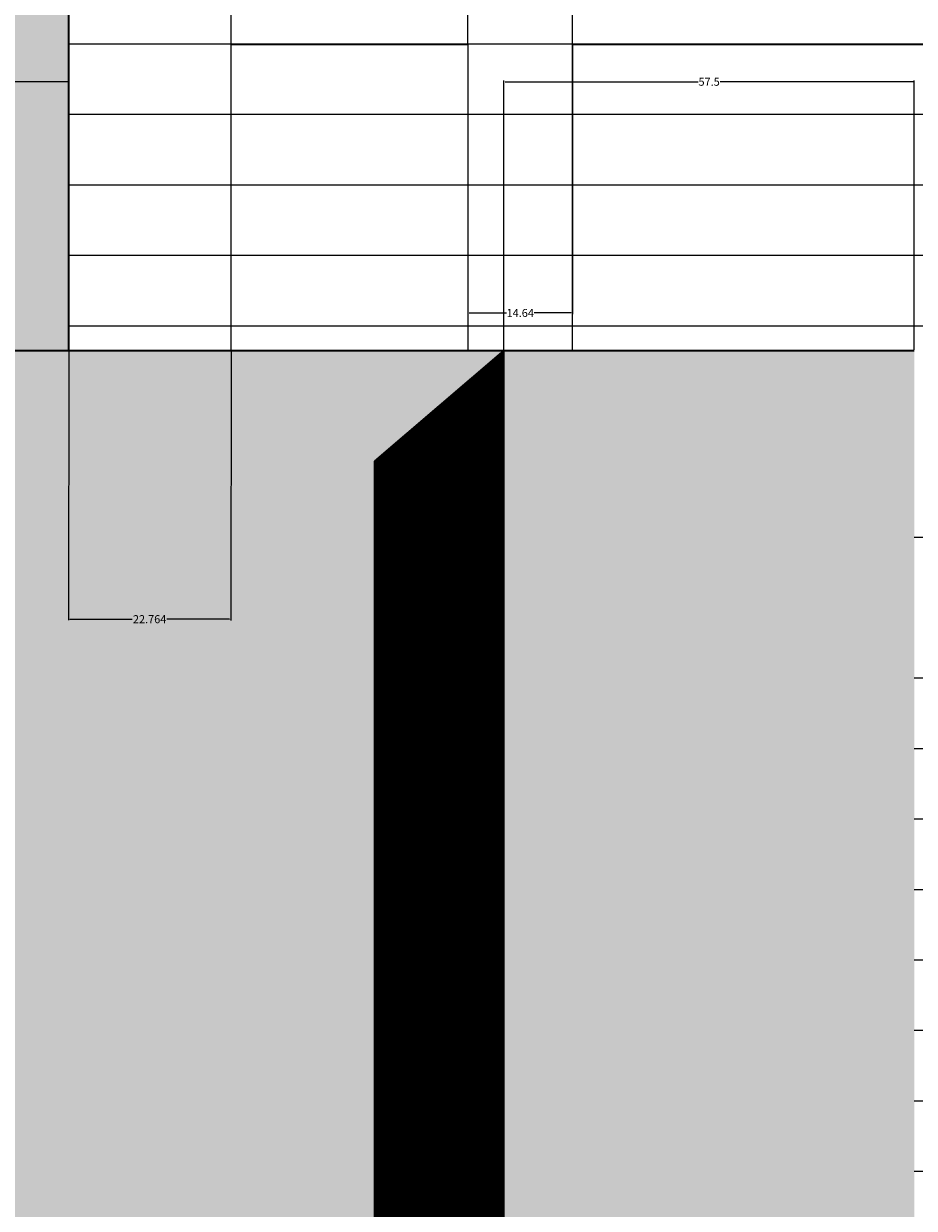
# Model space of a CAD drawing. Units: inches. Extents: x 8 to 634, y 41 to 867.
# Tile 18 of 21: x 293 to 418, y 577 to 743. Entities that reach past the tile are written whole.
import ezdxf

# ---------------------------------------------------------------- set-up
doc = ezdxf.new("R2010")
doc.units = ezdxf.units.IN
doc.header["$MEASUREMENT"] = 0
for name, color, linetype, lineweight in [('A-ANNO-DIMS', 2, 'Continuous', 18), ('A-ELEV-PATT', 252, 'Continuous', 9), ('A-GLAZ', 4, 'Continuous', 25), ('A-ROOF', 7, 'Continuous', 35), ('A-ROOF-PATT', 8, 'Continuous', 9), ('A-WALL', 7, 'Continuous', 35), ('A-WALL-PATT', 8, 'Continuous', 9)]:
    doc.layers.add(name, color=color, linetype=linetype, lineweight=lineweight)
doc.layers.add('A-GLAZ-PATT', color=251, linetype='Continuous', lineweight=9, true_color=0x636466)
doc.styles.get("Standard").update_dxf_attribs({"font": 'arial.ttf'})
doc.dimstyles.get("Standard").update_dxf_attribs({"dimtxt": 1.125, "dimasz": 0.18, "dimexe": 0.18, "dimexo": 0.0625, "dimgap": 0.09, "dimtad": 0, "dimtih": 1, "dimtoh": 1, "dimdec": 4, "dimzin": 0, "dimdsep": 46, "dimlunit": 4, "dimtxsty": 'Standard', "dimcen": 0.09, "dimadec": 0, "dimazin": 0, "dimtfac": 1, "dimtdec": 4, "dimtofl": 0, "dimtmove": 0, "dimatfit": 3, "dimfxl": 1, "dimtolj": 1, "dimtzin": 0, "dimarcsym": 0})

# ---------------------------------------------------------------- blocks, each defined once
blk = doc.blocks.new('*D19')
at = {"layer": 'A-ANNO-DIMS', "color": 0, "lineweight": -2, "transparency": 16777216}
for p, q in [((47.34, 697.73), (47.34, 866.81)), ((594.35, 827.83), (594.35, 866.81)), ((47.52, 866.63), (319.51, 866.63)), ((594.17, 866.63), (322.18, 866.63))]:
    blk.add_line(p, q, dxfattribs=at)
at = {"layer": 'A-ANNO-DIMS', "color": 0, "transparency": 16777216}
for points in [[(47.52, 866.66), (47.52, 866.6), (47.34, 866.63)], [(594.17, 866.66), (594.17, 866.6), (594.35, 866.63)]]:
    blk.add_solid(points, dxfattribs=at)
at = {"layer": 'Defpoints', "color": 0, "transparency": 16777216}
for p in [(594.35, 866.63), (594.35, 827.77), (47.34, 697.67)]:
    blk.add_point(p, dxfattribs=at)
at = {"layer": 'A-ANNO-DIMS', "color": 0, "transparency": 16777216, "insert": (320.85, 866.63), "char_height": 1.125, "attachment_point": 5}
blk.add_mtext('\\A1;547', dxfattribs=at)
blk = doc.blocks.new('*D24')
at = {"layer": 'A-ANNO-DIMS', "color": 0, "lineweight": -2, "transparency": 16777216}
for p, q in [((262.23, 697.73), (262.23, 735.5)), ((299.8, 697.73), (299.8, 735.5)), ((262.41, 735.32), (279.02, 735.32)), ((299.62, 735.32), (283, 735.32))]:
    blk.add_line(p, q, dxfattribs=at)
at = {"layer": 'A-ANNO-DIMS', "color": 0, "transparency": 16777216}
for points in [[(262.41, 735.35), (262.41, 735.29), (262.23, 735.32)], [(299.62, 735.35), (299.62, 735.29), (299.8, 735.32)]]:
    blk.add_solid(points, dxfattribs=at)
at = {"layer": 'Defpoints', "color": 0, "transparency": 16777216}
for p in [(299.8, 735.32), (262.23, 697.67), (299.8, 697.67)]:
    blk.add_point(p, dxfattribs=at)
at = {"layer": 'A-ANNO-DIMS', "color": 0, "transparency": 16777216, "insert": (281.01, 735.32), "char_height": 1.125, "attachment_point": 5}
blk.add_mtext('\\A1;37.57', dxfattribs=at)
blk = doc.blocks.new('*D25')
at = {"layer": 'A-ANNO-DIMS', "color": 0, "lineweight": -2, "transparency": 16777216}
for p, q in [((299.8, 697.6), (299.76, 659.84)), ((322.56, 697.58), (322.52, 659.81)), ((299.94, 660.02), (308.71, 660.01)), ((322.34, 659.99), (313.57, 660))]:
    blk.add_line(p, q, dxfattribs=at)
at = {"layer": 'A-ANNO-DIMS', "color": 0, "transparency": 16777216}
for points in [[(299.94, 660.05), (299.94, 659.99), (299.76, 660.02)], [(322.34, 660.02), (322.34, 659.96), (322.52, 659.99)]]:
    blk.add_solid(points, dxfattribs=at)
at = {"layer": 'Defpoints', "color": 0, "transparency": 16777216}
for p in [(299.8, 697.67), (322.56, 697.64), (299.76, 660.02)]:
    blk.add_point(p, dxfattribs=at)
at = {"layer": 'A-ANNO-DIMS', "color": 0, "transparency": 16777216, "insert": (311.14, 660), "char_height": 1.125, "attachment_point": 5}
blk.add_mtext('\\A1;22.764', dxfattribs=at)
blk = doc.blocks.new('*D48')
at = {"layer": 'A-ANNO-DIMS', "color": 0, "lineweight": -2, "transparency": 16777216}
for p, q in [((322.56, 740.62), (322.56, 778.39)), ((322.74, 778.21), (336.73, 778.21)), ((355.57, 778.21), (341.58, 778.21)), ((355.75, 740.62), (355.75, 778.39))]:
    blk.add_line(p, q, dxfattribs=at)
at = {"layer": 'A-ANNO-DIMS', "color": 0, "transparency": 16777216}
for points in [[(322.74, 778.24), (322.74, 778.18), (322.56, 778.21)], [(355.57, 778.24), (355.57, 778.18), (355.75, 778.21)]]:
    blk.add_solid(points, dxfattribs=at)
at = {"layer": 'Defpoints', "color": 0, "transparency": 16777216}
for p in [(355.75, 778.21), (322.56, 740.56), (355.75, 740.56)]:
    blk.add_point(p, dxfattribs=at)
at = {"layer": 'A-ANNO-DIMS', "color": 0, "transparency": 16777216, "insert": (339.15, 778.21), "char_height": 1.125, "attachment_point": 5}
blk.add_mtext('\\A1;33.187', dxfattribs=at)
blk = doc.blocks.new('*D49')
at = {"layer": 'A-ANNO-DIMS', "color": 0, "lineweight": -2, "transparency": 16777216}
for p, q in [((355.75, 740.49), (355.75, 702.73)), ((370.39, 740.49), (370.39, 702.73)), ((355.93, 702.91), (361.13, 702.91)), ((370.21, 702.91), (365, 702.91))]:
    blk.add_line(p, q, dxfattribs=at)
at = {"layer": 'A-ANNO-DIMS', "color": 0, "transparency": 16777216}
for points in [[(355.93, 702.94), (355.93, 702.88), (355.75, 702.91)], [(370.21, 702.94), (370.21, 702.88), (370.39, 702.91)]]:
    blk.add_solid(points, dxfattribs=at)
at = {"layer": 'Defpoints', "color": 0, "transparency": 16777216}
for p in [(355.75, 740.56), (370.39, 740.56), (355.75, 702.91)]:
    blk.add_point(p, dxfattribs=at)
at = {"layer": 'A-ANNO-DIMS', "color": 0, "transparency": 16777216, "insert": (363.07, 702.91), "char_height": 1.125, "attachment_point": 5}
blk.add_mtext('\\A1;14.64', dxfattribs=at)
blk = doc.blocks.new('*D50')
at = {"layer": 'A-ANNO-DIMS', "color": 0, "lineweight": -2, "transparency": 16777216}
for p, q in [((370.39, 740.62), (370.39, 778.39)), ((370.57, 778.21), (402.91, 778.21)), ((439.02, 778.21), (406.68, 778.21)), ((439.2, 740.62), (439.2, 778.39))]:
    blk.add_line(p, q, dxfattribs=at)
at = {"layer": 'A-ANNO-DIMS', "color": 0, "transparency": 16777216}
for points in [[(370.57, 778.24), (370.57, 778.18), (370.39, 778.21)], [(439.02, 778.24), (439.02, 778.18), (439.2, 778.21)]]:
    blk.add_solid(points, dxfattribs=at)
at = {"layer": 'Defpoints', "color": 0, "transparency": 16777216}
for p in [(439.2, 778.21), (370.39, 740.56), (439.2, 740.56)]:
    blk.add_point(p, dxfattribs=at)
at = {"layer": 'A-ANNO-DIMS', "color": 0, "transparency": 16777216, "insert": (404.79, 778.21), "char_height": 1.125, "attachment_point": 5}
blk.add_mtext('\\A1;68.81', dxfattribs=at)
blk = doc.blocks.new('*D63')
at = {"layer": 'A-ANNO-DIMS', "color": 0, "lineweight": -2, "transparency": 16777216}
for p, q in [((360.79, 697.73), (360.79, 735.5)), ((418.29, 697.73), (418.29, 735.5)), ((360.97, 735.32), (387.98, 735.32)), ((418.11, 735.32), (391.09, 735.32))]:
    blk.add_line(p, q, dxfattribs=at)
at = {"layer": 'A-ANNO-DIMS', "color": 0, "transparency": 16777216}
for points in [[(360.97, 735.35), (360.97, 735.29), (360.79, 735.32)], [(418.11, 735.35), (418.11, 735.29), (418.29, 735.32)]]:
    blk.add_solid(points, dxfattribs=at)
at = {"layer": 'Defpoints', "color": 0, "transparency": 16777216}
for p in [(418.29, 735.32), (360.79, 697.67), (418.29, 697.67)]:
    blk.add_point(p, dxfattribs=at)
at = {"layer": 'A-ANNO-DIMS', "color": 0, "transparency": 16777216, "insert": (389.54, 735.32), "char_height": 1.125, "attachment_point": 5}
blk.add_mtext('\\A1;57.5', dxfattribs=at)

msp = doc.modelspace()

# ---------------------------------------------------------------- hatches: boundary and pattern name
at = {"layer": 'A-ELEV-PATT', "transparency": 33554544}
h = msp.add_hatch(dxfattribs=at)
h.set_pattern_fill('ANSI31', color=256)
h.paths.add_polyline_path([(360.785, 697.6655), (342.6544, 682.1444), (342.6544, 569.1705), (360.785, 569.1705)])
h.paths.add_polyline_path([(360.785, 523.5555), (360.785, 569.1705), (342.6544, 569.1705), (342.6544, 449.7533), (360.785, 449.7533)])
h.paths.add_polyline_path([(360.785, 449.7533), (342.6544, 449.7533), (342.6544, 391.7598), (360.785, 391.7598)])
h.paths.add_polyline_path([(360.785, 391.7598), (342.6544, 391.7598), (342.6544, 272.3426), (360.785, 272.3426)])
h.paths.add_polyline_path([(360.785, 272.3426), (342.6544, 272.3426), (342.6544, 235.5555), (360.785, 235.5555)])
h.paths.add_polyline_path([(360.785, 235.5555), (342.6544, 235.5555), (342.6544, 224.3257), (353.4573, 224.3257), (353.4573, 101.0012), (342.6544, 101.0012), (342.6544, 91.5417), (360.785, 91.5417)])
at = {"layer": 'A-GLAZ-PATT', "transparency": 33554687}
h = msp.add_hatch(dxfattribs=at)
h.set_pattern_fill('ANSI31', color=256, scale=79, angle=135)
h.paths.add_polyline_path([(355.7466, 740.5561), (322.56, 740.5561), (322.56, 697.6655), (355.7466, 697.6655)])
h.paths.add_polyline_path([(439.201, 740.5561), (370.3877, 740.5561), (370.3877, 697.6655), (418.2881, 697.6655), (418.2881, 691.978), (439.201, 691.978)])
h.paths.add_polyline_path([(498.2535, 740.5561), (449.4498, 740.5561), (449.4498, 691.978), (498.2535, 691.978)])
h.paths.add_polyline_path([(536.3204, 740.5561), (508.5023, 740.5561), (508.5023, 691.978), (536.3204, 691.978)])
h.paths.add_polyline_path([(439.201, 690.978), (418.2881, 690.978), (418.2881, 682.0586), (439.201, 682.0586)])
h.paths.add_polyline_path([(439.201, 681.0586), (418.2881, 681.0586), (418.2881, 673.2414), (439.201, 673.2414)])
h.paths.add_polyline_path([(439.201, 672.2414), (418.2881, 672.2414), (418.2881, 662.4168), (439.201, 662.4168)])
h.paths.add_polyline_path([(439.201, 661.4168), (418.2881, 661.4168), (418.2881, 651.537), (439.201, 651.537)])
h.paths.add_polyline_path([(439.201, 650.537), (418.2881, 650.537), (418.2881, 640.7358), (439.201, 640.7358)])
h.paths.add_polyline_path([(439.201, 639.7358), (418.2881, 639.7358), (418.2881, 630.9186), (439.201, 630.9186)])
h.paths.add_polyline_path([(439.201, 629.9186), (418.2881, 629.9186), (418.2881, 619.6298), (439.201, 619.6298)])
h.paths.add_polyline_path([(477.6441, 629.9186), (449.4498, 629.9186), (449.4498, 619.6298), (477.6441, 619.6298)])
h.paths.add_polyline_path([(477.6441, 639.7358), (449.4498, 639.7358), (449.4498, 630.9186), (477.6441, 630.9186)])
h.paths.add_polyline_path([(477.6441, 650.537), (449.4498, 650.537), (449.4498, 640.7358), (477.6441, 640.7358)])
h.paths.add_polyline_path([(477.6441, 661.4168), (449.4498, 661.4168), (449.4498, 651.537), (477.6441, 651.537)])
h.paths.add_polyline_path([(477.6441, 672.2414), (449.4498, 672.2414), (449.4498, 662.4168), (477.6441, 662.4168)])
h.paths.add_polyline_path([(477.6441, 681.0586), (449.4498, 681.0586), (449.4498, 673.2414), (477.6441, 673.2414)])
h.paths.add_polyline_path([(477.6441, 690.978), (449.4498, 690.978), (449.4498, 682.0586), (477.6441, 682.0586)])
h.paths.add_polyline_path([(498.2535, 690.978), (478.6441, 690.978), (478.6441, 682.0586), (498.2535, 682.0586)])
h.paths.add_polyline_path([(498.2535, 681.0586), (478.6441, 681.0586), (478.6441, 673.2414), (498.2535, 673.2414)])
h.paths.add_polyline_path([(498.2535, 672.2414), (478.6441, 672.2414), (478.6441, 662.4168), (498.2535, 662.4168)])
h.paths.add_polyline_path([(498.2535, 661.4168), (478.6441, 661.4168), (478.6441, 651.537), (498.2535, 651.537)])
h.paths.add_polyline_path([(498.2535, 650.537), (478.6441, 650.537), (478.6441, 640.7358), (498.2535, 640.7358)])
h.paths.add_polyline_path([(498.2535, 639.7358), (478.6441, 639.7358), (478.6441, 630.9186), (498.2535, 630.9186)])
h.paths.add_polyline_path([(498.2535, 629.9186), (478.6441, 629.9186), (478.6441, 619.6298), (498.2535, 619.6298)])
h.paths.add_polyline_path([(536.3204, 629.9186), (508.5023, 629.9186), (508.5023, 619.6298), (536.3204, 619.6298)])
h.paths.add_polyline_path([(536.3204, 639.7358), (508.5023, 639.7358), (508.5023, 630.9186), (536.3204, 630.9186)])
h.paths.add_polyline_path([(536.3204, 650.537), (508.5023, 650.537), (508.5023, 640.7358), (536.3204, 640.7358)])
h.paths.add_polyline_path([(536.3204, 661.4168), (508.5023, 661.4168), (508.5023, 651.537), (536.3204, 651.537)])
h.paths.add_polyline_path([(536.3204, 672.2414), (508.5023, 672.2414), (508.5023, 662.4168), (536.3204, 662.4168)])
h.paths.add_polyline_path([(536.3204, 681.0586), (508.5023, 681.0586), (508.5023, 673.2414), (536.3204, 673.2414)])
h.paths.add_polyline_path([(536.3204, 690.978), (508.5023, 690.978), (508.5023, 682.0586), (536.3204, 682.0586)])
h.paths.add_polyline_path([(342.6544, 175.7749), (302.6522, 224.3257), (302.6522, 101.0012), (342.6544, 149.552)])
h.paths.add_polyline_path([(342.6544, 224.3257), (302.6522, 224.3257), (342.6544, 175.7749)])
h.paths.add_polyline_path([(342.6544, 149.552), (302.6522, 101.0012), (342.6544, 101.0012)])
h.paths.add_polyline_path([(353.4573, 162.6634), (342.6544, 149.552), (342.6544, 101.0012), (353.4573, 101.0012)])
h.paths.add_polyline_path([(353.4573, 224.3257), (342.6544, 224.3257), (342.6544, 101.0012), (353.4573, 101.0012)])
h.paths.add_polyline_path([(342.6544, 175.7749), (342.6544, 149.552), (353.4573, 162.6634)], flags=17)
at = {"layer": 'A-ROOF-PATT', "transparency": 33554687}
h = msp.add_hatch(dxfattribs=at)
h.set_pattern_fill('AR-CONC', color=256, scale=2.2, angle=135)
h.paths.add_polyline_path([(262.2266, 828.9821), (144.3564, 828.9821), (144.3564, 697.6655), (262.2266, 785.231), (245.114, 785.231), (245.114, 792.8938), (262.2266, 792.8938)])
h.paths.add_polyline_path([(594.3501, 827.7671), (262.2266, 827.7671), (262.2266, 792.8938), (262.2266, 697.6655), (299.7961, 697.6655), (299.7961, 776.8929), (556.7072, 776.8929), (556.7072, 774.3342), (556.7072, 697.6655), (594.3501, 697.6655)])
at = {"layer": 'A-WALL-PATT', "transparency": 33554687}
h = msp.add_hatch(dxfattribs=at)
h.set_pattern_fill('ANSI31', color=256, scale=79, angle=135)
h.paths.add_polyline_path([(539.0002, 276.166), (499.4677, 276.166), (418.2881, 276.166), (418.2881, 228.4951), (435.5682, 228.4951), (539.0002, 228.4951)])
h.paths.add_polyline_path([(539.0002, 228.4951), (435.5682, 228.4951), (418.2881, 228.4951), (418.2881, 112.2342), (439.3242, 112.2342), (539.0002, 112.2342)])
h.paths.add_polyline_path([(518.1129, 124.2342), (473.3277, 124.2342), (473.3277, 216.4951), (518.1129, 216.4951)], flags=16)
h.paths.add_polyline_path([(451.2116, 124.2342), (427.4368, 124.2342), (427.4368, 216.4951), (451.2116, 216.4951)], flags=16)
h.paths.add_polyline_path([(539.0002, 112.2342), (439.3242, 112.2342), (418.2881, 112.2342), (418.2881, 91.5417), (539.0002, 91.5417)])
h.paths.add_polyline_path([(539.0002, 392.4268), (427.4368, 392.4268), (418.2881, 392.4268), (418.2881, 391.7598), (418.2881, 276.166), (499.4677, 276.166), (539.0002, 276.166)])
h.paths.add_polyline_path([(518.1129, 288.166), (473.3277, 288.166), (473.3277, 380.4268), (518.1129, 380.4268)], flags=16)
h.paths.add_polyline_path([(451.2116, 288.166), (427.4368, 288.166), (427.4368, 380.4268), (451.2116, 380.4268)], flags=16)
h.paths.add_polyline_path([(539.0002, 451.6305), (427.4368, 452.9097), (418.2881, 452.9097), (418.2881, 392.4268), (427.4368, 392.4268), (539.0002, 392.4268)])
h.paths.add_polyline_path([(539.0002, 569.1705), (427.4368, 569.1705), (418.2881, 569.1705), (418.2881, 452.9097), (427.4368, 452.9097), (539.0002, 451.6305)])
h.paths.add_polyline_path([(473.3277, 557.1705), (518.1129, 557.1705), (518.1129, 464.9097), (473.3277, 464.9097)], flags=16)
h.paths.add_polyline_path([(451.2116, 557.1705), (451.2116, 464.9097), (427.4368, 464.9097), (427.4368, 557.1705)], flags=16)
h.paths.add_polyline_path([(539.0002, 619.6298), (418.2881, 619.6298), (418.2881, 569.1705), (427.4368, 569.1705), (539.0002, 569.1705)])
h.paths.add_polyline_path([(556.7072, 774.3342), (556.7072, 776.8929), (299.7961, 776.8929), (299.7961, 697.6655), (322.56, 697.6655), (322.56, 740.5561), (355.7466, 740.5561), (355.7466, 697.6655), (360.785, 697.6655), (370.3877, 697.6655), (370.3877, 740.5561), (439.201, 740.5561), (439.201, 691.978), (449.4498, 691.978), (449.4498, 740.5561), (498.2535, 740.5561), (498.2535, 691.978), (508.5023, 691.978), (508.5023, 740.5561), (536.3204, 740.5561), (536.3204, 691.978), (539.0002, 691.978), (539.0002, 697.6655), (556.7072, 697.6655)])
h = msp.add_hatch(dxfattribs=at)
h.set_pattern_fill('AR-CONC', color=256, scale=3.2)
h.paths.add_polyline_path([(119.7065, 697.6655), (47.3401, 697.6655), (47.3401, 569.1705), (119.7065, 569.1705)])
h.paths.add_polyline_path([(202.1558, 697.6655), (119.7065, 697.6655), (119.7065, 569.1705), (202.1558, 569.1705)])
h.paths.add_polyline_path([(284.6051, 697.6655), (202.1558, 697.6655), (202.1558, 569.1705), (284.6051, 569.1705)])
h.paths.add_polyline_path([(119.7065, 569.1705), (47.3401, 569.1705), (47.3401, 523.5555), (47.3401, 449.7533), (119.7065, 449.7533)])
h.paths.add_polyline_path([(342.6544, 682.1444), (360.785, 697.6655), (284.6051, 697.6655), (284.6051, 569.1705), (342.6544, 569.1705)])
h.paths.add_polyline_path([(342.6544, 569.1705), (284.6051, 569.1705), (284.6051, 449.7533), (342.6544, 449.7533)])
h.paths.add_polyline_path([(418.2881, 691.978), (418.2881, 697.6655), (360.785, 697.6655), (360.785, 569.1705), (418.2881, 569.1705)])
h.paths.add_polyline_path([(418.2881, 569.1705), (360.785, 569.1705), (360.785, 523.5555), (360.785, 449.7533), (418.2881, 449.7533)])
h.paths.add_polyline_path([(594.3501, 697.6655), (539.0002, 697.6655), (539.0002, 691.978), (539.0002, 569.1705), (594.3501, 569.1705)])
h.paths.add_polyline_path([(594.3501, 523.5555), (594.3501, 569.1705), (539.0002, 569.1705), (539.0002, 451.6305), (594.3501, 451.6305)])
h.paths.add_polyline_path([(594.3501, 451.6305), (539.0002, 451.6305), (539.0002, 391.7598), (594.3501, 391.7598)])
h.paths.add_polyline_path([(594.3501, 391.7598), (539.0002, 391.7598), (539.0002, 276.166), (594.3501, 276.166)])
h.paths.add_polyline_path([(418.2881, 449.7533), (360.785, 449.7533), (360.785, 391.7598), (418.2881, 391.7598)])
h.paths.add_polyline_path([(342.6544, 449.7533), (284.6051, 449.7533), (284.6051, 391.7598), (342.6544, 391.7598)])
h.paths.add_polyline_path([(342.6544, 391.7598), (284.6051, 391.7598), (284.6051, 272.3426), (342.6544, 272.3426)])
h.paths.add_polyline_path([(418.2881, 391.7598), (360.785, 391.7598), (360.785, 272.3426), (418.2881, 272.3426)])
h.paths.add_polyline_path([(418.2881, 272.3426), (360.785, 272.3426), (360.785, 235.5555), (418.2881, 235.5555)])
h.paths.add_polyline_path([(342.6544, 272.3426), (284.6051, 272.3426), (284.6051, 235.5555), (295.0049, 235.5555), (342.6544, 235.5555)])
h.paths.add_polyline_path([(594.3501, 276.166), (539.0002, 276.166), (539.0002, 228.4951), (594.3501, 228.4951)])
h.paths.add_polyline_path([(594.3501, 228.4951), (539.0002, 228.4951), (539.0002, 91.5417), (594.3501, 91.5417)])
h.paths.add_polyline_path([(418.2881, 235.5555), (360.785, 235.5555), (360.785, 91.5417), (418.2881, 91.5417)])
h.paths.add_polyline_path([(284.6051, 272.3426), (119.7065, 272.3426), (119.7065, 235.5555), (284.6051, 235.5555)])
h.paths.add_polyline_path([(119.7065, 272.3426), (47.3401, 272.3426), (47.3401, 235.5555), (47.3401, 91.5555), (63.5448, 91.5555), (63.5448, 227.8036), (268.998, 227.8036), (268.998, 91.5555), (295.0049, 91.5555), (295.0049, 222.583), (271.9787, 222.583), (271.9787, 229.0481), (62.4019, 229.0481), (62.4019, 222.583), (61.1827, 222.583), (61.1827, 235.5555), (119.7065, 235.5555)])
h.paths.add_polyline_path([(119.7065, 391.7598), (47.3401, 391.7598), (47.3401, 379.5555), (47.3401, 272.3426), (119.7065, 272.3426)])
h.paths.add_polyline_path([(119.7065, 449.7533), (47.3401, 449.7533), (47.3401, 391.7598), (119.7065, 391.7598)])
h.paths.add_polyline_path([(202.1558, 449.7533), (119.7065, 449.7533), (119.7065, 391.7598), (202.1558, 391.7598)])
h.paths.add_polyline_path([(284.6051, 449.7533), (202.1558, 449.7533), (202.1558, 391.7598), (284.6051, 391.7598)])

# ---------------------------------------------------------------- linework, layer by layer
at = {"layer": 'A-GLAZ'}
for p, q in [((322.56, 697.6432), (322.56, 740.5561)), ((322.56, 740.5561), (355.7466, 740.5561)), ((355.7466, 740.5561), (355.7466, 697.6655)), ((370.3877, 697.6655), (370.3877, 740.5561)), ((370.3877, 740.5561), (439.201, 740.5561))]:
    msp.add_line(p, q, dxfattribs=at)
at = {"layer": 'A-ROOF'}
msp.add_line((299.7961, 697.6655), (299.7961, 776.8929), dxfattribs=at)
at = {"layer": 'A-WALL'}
for p, q in [((47.3401, 697.6655), (360.785, 697.6655)), ((360.785, 697.6655), (342.6544, 682.1444)), ((360.785, 523.5555), (360.785, 697.6655)), ((360.785, 697.6655), (418.2881, 697.6655)), ((342.6544, 682.1444), (342.6544, 91.5555))]:
    msp.add_line(p, q, dxfattribs=at)

# ---------------------------------------------------------------- dimensions: what is measured, and where the dimension line sits
at = {"layer": 'A-ANNO-DIMS'}
for base, p1, p2, override, picture, middle in [((594.3501, 866.6321), (47.3401, 697.6655), (594.3501, 827.7671), {"dimdec": 0, "dimlfac": 1, "dimrnd": 0, "dimzin": 0, "dimdsep": 46, "dimlunit": 2}, '*D19', (320.8451, 866.6321)), ((355.7466, 778.2061), (322.56, 740.5561), (355.7466, 740.5561), {"dimdec": 3, "dimlfac": 1, "dimrnd": 0, "dimzin": 0, "dimdsep": 46, "dimlunit": 2}, '*D48', (339.1533, 778.2061)), ((439.201, 778.2061), (370.3877, 740.5561), (439.201, 740.5561), {"dimdec": 2, "dimlfac": 1, "dimrnd": 0, "dimzin": 0, "dimdsep": 46, "dimlunit": 2}, '*D50', (404.7943, 778.2061)), ((299.7961, 735.3155), (262.2266, 697.6655), (299.7961, 697.6655), {"dimdec": 2, "dimlfac": 1, "dimrnd": 0, "dimzin": 0, "dimdsep": 46, "dimlunit": 2}, '*D24', (281.0113, 735.3155)), ((418.2881, 735.3155), (360.785, 697.6655), (418.2881, 697.6655), {"dimdec": 1, "dimlfac": 1, "dimrnd": 0, "dimzin": 0, "dimdsep": 46, "dimlunit": 2}, '*D63', (389.5366, 735.3155))]:
    dim = msp.add_linear_dim(base=base, p1=p1, p2=p2, dimstyle='Standard', override=override, dxfattribs=at)
    dim.commit()
    dim.dimension.update_dxf_attribs({"geometry": picture, "text_midpoint": middle})
for base, p1, p2, angle, override, picture, middle in [((355.7466, 702.9061), (370.3877, 740.5561), (355.7466, 740.5561), 180, {"dimdec": 2, "dimlfac": 1, "dimrnd": 0, "dimzin": 0, "dimdsep": 46, "dimlunit": 2}, '*D49', (363.0671, 702.9061)), ((299.7591, 660.0156), (322.56, 697.6432), (299.7961, 697.6655), 179.943826, {"dimdec": 3, "dimlfac": 1, "dimrnd": 0, "dimzin": 0, "dimdsep": 46, "dimlunit": 2}, '*D25', (311.1411, 660.0044))]:
    dim = msp.add_linear_dim(base=base, p1=p1, p2=p2, angle=angle, dimstyle='Standard', override=override, dxfattribs=at)
    dim.commit()
    dim.dimension.update_dxf_attribs({"geometry": picture, "text_midpoint": middle})

doc.saveas('drawing.dxf')
